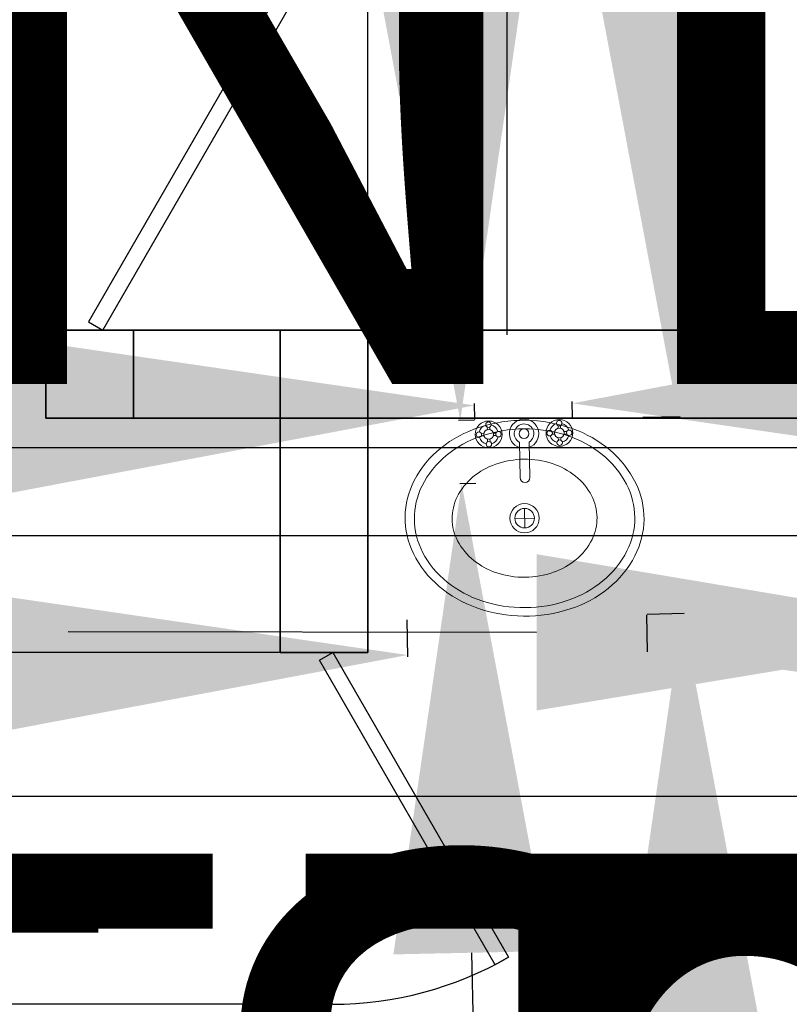
# Model space of a CAD drawing. Units: inches. Extents: x -307 to 2141, y -58 to 895.
# Tile 21 of 28: x 776 to 855, y 481 to 582. Entities that reach past the tile are written whole.
import ezdxf

# ---------------------------------------------------------------- set-up
doc = ezdxf.new("R2010")
doc.units = ezdxf.units.IN
doc.header["$MEASUREMENT"] = 0
for name, color, linetype, lineweight in [('A-ANNO-DIMS', 2, 'Continuous', 18), ('A-DOOR', 3, 'Continuous', 25), ('A-FLOR-FIXT', 9, 'Continuous', 18), ('A-WALL', 7, 'Continuous', 35)]:
    doc.layers.add(name, color=color, linetype=linetype, lineweight=lineweight)
doc.styles.get("Standard").update_dxf_attribs({"font": 'arial.ttf'})
doc.dimstyles.get("Standard").update_dxf_attribs({"dimtxt": 72, "dimasz": 48, "dimexe": 0.18, "dimexo": 0.0625, "dimgap": 0.09, "dimtad": 0, "dimtih": 1, "dimtoh": 1, "dimdec": 0, "dimrnd": 48, "dimzin": 0, "dimdsep": 46, "dimlunit": 3, "dimtxsty": 'Standard', "dimcen": 0.09, "dimadec": 0, "dimazin": 0, "dimtfac": 1, "dimtdec": 0, "dimtofl": 0, "dimtmove": 0, "dimatfit": 3, "dimfxl": 1, "dimtolj": 1, "dimtzin": 0, "dimarcsym": 0})

# ---------------------------------------------------------------- blocks, each defined once
blk = doc.blocks.new('*U2')
for p, q in [((0, 0), (0, -6)), ((-40, 0), (-40, -6))]:
    blk.add_line(p, q)
blk.add_lwpolyline([(0, 0), (-34.64, 20), (-35.52, 18.48), (-0.87, -1.52)], close=True)
blk.add_arc((0, 0), 40, 150, 180)
blk = doc.blocks.new('*U4')
for p, q in [((-40, 0), (-40, 6)), ((0, 0), (0, 6))]:
    blk.add_line(p, q)
blk.add_lwpolyline([(0, 0), (-34.64, -20), (-35.52, -18.48), (-0.88, 1.52)], close=True)
blk.add_arc((0, 0), 40, 180, 210)
blk = doc.blocks.new('Faucet - Bathroom top')
for p, q in [((-4.107, 0.125), (-4.375, 0.125)), ((-3.75, 0.4788), (-3.75, 0.75)), ((-3.5, 0.482), (-3.5, 0.75)), ((-3.1461, 0.125), (-2.875, 0.125)), ((3.143, 0.125), (2.875, 0.125)), ((3.5, 0.4788), (3.5, 0.75)), ((3.75, 0.482), (3.75, 0.75)), ((4.1039, 0.125), (4.375, 0.125)), ((-4.1039, -0.125), (-4.375, -0.125)), ((-3.75, -0.4821), (-3.75, -0.75)), ((-3.5, -0.4789), (-3.5, -0.75)), ((-3.143, -0.125), (-2.875, -0.125)), ((-0.5, -0.8639), (-0.5, -4.5)), ((0.5, -4.5), (0.5, -0.8631)), ((3.1461, -0.125), (2.875, -0.125)), ((3.5, -0.4821), (3.5, -0.75)), ((3.75, -0.4789), (3.75, -0.75)), ((4.107, -0.125), (4.375, -0.125))]:
    blk.add_line(p, q)
for centre, radius in [((-3.625, 0), 1.375), ((-3.625, 1), 0.2795), ((3.625, 0), 1.375), ((3.625, 1), 0.2795), ((-4.625, 0), 0.2795), ((-3.625, 0), 0.5), ((-2.625, 0), 0.2795), ((0, 0), 0.5), ((2.625, 0), 0.2795), ((3.625, 0), 0.5), ((4.625, 0), 0.2795), ((-3.625, -1), 0.2795), ((3.625, -1), 0.2795)]:
    blk.add_circle(centre, radius)
for centre, radius, start, end in [((0, 0), 1.5, 289.6514, 250.3603), ((-3.625, 0), 1, 105.2407, 164.2093), ((-3.625, 0), 1, 16.44125, 74.07887), ((0, 0), 1, 300.3431, 239.7554), ((3.625, 0), 1, 106.12, 164.0884), ((3.625, 0), 1, 16.23422, 73.90469), ((-3.625, 0), 1, 196.2342, 253.9047), ((-3.625, 0), 1, 286.12, 344.0884), ((3.625, 0), 1, 196.4413, 254.0789), ((3.625, 0), 1, 285.2407, 344.2093), ((0, -4.5), 0.5, 180, 0)]:
    blk.add_arc(centre, radius, start, end)
blk = doc.blocks.new('Sink - Oval top')
for p, q in [((-1, 0), (1, 0)), ((0, 1), (0, -1))]:
    blk.add_line(p, q)
for points in [[(-12.23, 0.39, 0.117634), (-11.46, -3.36, 0.104469), (-8.88, -6.8, 0.090016), (-5.08, -9.07, 0.08192), (-0.32, -10.02, 0.08192), (4.49, -9.38, 0.090016), (8.42, -7.36, 0.104469), (11.22, -4.09, 0.117634), (12.23, -0.39, 0.117634), (11.46, 3.36, 0.104469), (8.88, 6.8, 0.090016), (5.08, 9.07, 0.08192), (0.32, 10.02, 0.08192), (-4.49, 9.38, 0.090016), (-8.42, 7.36, 0.104469), (-11.22, 4.09, 0.117634)], [(-11.29, 0.16, 0.118622), (-10.52, -3.25, 0.104678), (-8.07, -6.36, 0.089562), (-4.54, -8.37, 0.081185), (-0.13, -9.15, 0.081185), (4.3, -8.49, 0.089562), (7.89, -6.58, 0.104678), (10.42, -3.55, 0.118622), (11.29, -0.16, 0.118622), (10.52, 3.25, 0.104678), (8.07, 6.36, 0.089562), (4.54, 8.37, 0.081185), (0.13, 9.15, 0.081185), (-4.3, 8.49, 0.089562), (-7.89, 6.58, 0.104678), (-10.42, 3.55, 0.118622)], [(-7.42, 0.08, 0.118283), (-6.91, -2.17, 0.104607), (-5.29, -4.21, 0.089718), (-2.97, -5.53, 0.081436), (-0.07, -6.04, 0.081436), (2.84, -5.59, 0.089718), (5.2, -4.33, 0.104607), (6.86, -2.32, 0.118283), (7.42, -0.08, 0.118283), (6.91, 2.17, 0.104607), (5.29, 4.21, 0.089718), (2.97, 5.53, 0.081436), (0.07, 6.04, 0.081436), (-2.84, 5.59, 0.089718), (-5.2, 4.33, 0.104607), (-6.86, 2.32, 0.118283)]]:
    blk.add_lwpolyline(points, format="xyb", close=True)
for radius in [1.5, 1]:
    blk.add_circle((0, 0), radius)
blk = doc.blocks.new('*D29')
at = {"layer": 'A-ANNO-DIMS', "color": 0, "lineweight": -2, "transparency": 16777216}
for p, q in [((747.42, 450.87), (699.42, 450.87)), ((795.42, 433.61), (795.42, 451.05)), ((882.03, 433.61), (882.03, 451.05)), ((930.03, 450.87), (978.03, 450.87))]:
    blk.add_line(p, q, dxfattribs=at)
at = {"layer": 'A-ANNO-DIMS', "color": 0, "transparency": 16777216}
for points in [[(747.42, 458.87), (747.42, 442.87), (795.42, 450.87)], [(930.03, 458.87), (930.03, 442.87), (882.03, 450.87)]]:
    blk.add_solid(points, dxfattribs=at)
at = {"layer": 'Defpoints', "color": 0, "transparency": 16777216}
for p in [(795.42, 450.87), (795.42, 433.55), (882.03, 433.55)]:
    blk.add_point(p, dxfattribs=at)
at = {"layer": 'A-ANNO-DIMS', "color": 0, "transparency": 16777216, "insert": (647.71, 450.87), "char_height": 72, "attachment_point": 5}
blk.add_mtext('\\A1;87', dxfattribs=at)
blk = doc.blocks.new('*D30')
at = {"layer": 'A-ANNO-DIMS', "color": 0, "lineweight": -2, "transparency": 16777216}
for p, q in [((570.74, 532.83), (570.74, 580.83)), ((570.74, 580.83), (618.74, 580.83)), ((565.4, 484.83), (570.92, 484.83)), ((565.4, 448.83), (570.92, 448.83)), ((570.74, 400.83), (570.74, 352.83))]:
    blk.add_line(p, q, dxfattribs=at)
at = {"layer": 'A-ANNO-DIMS', "color": 0, "transparency": 16777216}
for points in [[(562.74, 532.83), (578.74, 532.83), (570.74, 484.83)], [(562.74, 400.83), (578.74, 400.83), (570.74, 448.83)]]:
    blk.add_solid(points, dxfattribs=at)
at = {"layer": 'Defpoints', "color": 0, "transparency": 16777216}
for p in [(565.34, 484.83), (570.74, 484.83), (565.34, 448.83)]:
    blk.add_point(p, dxfattribs=at)
at = {"layer": 'A-ANNO-DIMS', "color": 0, "transparency": 16777216, "insert": (1030.17, 580.83), "char_height": 72, "attachment_point": 5}
blk.add_mtext('\\A1;WINDOW 36 TYP.', dxfattribs=at)
blk = doc.blocks.new('*D31')
at = {"layer": 'A-ANNO-DIMS', "color": 0, "lineweight": -2, "transparency": 16777216}
for p, q in [((556.34, 448.77), (556.34, 443.25)), ((565.34, 448.77), (565.34, 443.25)), ((508.34, 443.43), (460.34, 443.43)), ((613.34, 443.43), (661.34, 443.43))]:
    blk.add_line(p, q, dxfattribs=at)
at = {"layer": 'A-ANNO-DIMS', "color": 0, "transparency": 16777216}
for points in [[(508.34, 451.43), (508.34, 435.43), (556.34, 443.43)], [(613.34, 451.43), (613.34, 435.43), (565.34, 443.43)]]:
    blk.add_solid(points, dxfattribs=at)
at = {"layer": 'Defpoints', "color": 0, "transparency": 16777216}
for p in [(556.34, 448.83), (565.34, 448.83), (565.34, 443.43)]:
    blk.add_point(p, dxfattribs=at)
at = {"layer": 'A-ANNO-DIMS', "color": 0, "transparency": 16777216, "insert": (808.69, 443.43), "char_height": 72, "attachment_point": 5}
blk.add_mtext('\\A1;9 TYP.', dxfattribs=at)
blk = doc.blocks.new('*D32')
at = {"layer": 'A-ANNO-DIMS', "color": 0, "lineweight": -2, "transparency": 16777216}
for p, q in [((813.29, 682.28), (813.29, 671.36)), ((885.29, 682.28), (885.29, 671.36)), ((765.29, 671.54), (717.29, 671.54)), ((933.29, 671.54), (981.29, 671.54))]:
    blk.add_line(p, q, dxfattribs=at)
at = {"layer": 'A-ANNO-DIMS', "color": 0, "transparency": 16777216}
for points in [[(765.29, 679.54), (765.29, 663.54), (813.29, 671.54)], [(933.29, 679.54), (933.29, 663.54), (885.29, 671.54)]]:
    blk.add_solid(points, dxfattribs=at)
at = {"layer": 'Defpoints', "color": 0, "transparency": 16777216}
for p in [(813.29, 682.34), (885.29, 682.34), (885.29, 671.54)]:
    blk.add_point(p, dxfattribs=at)
at = {"layer": 'A-ANNO-DIMS', "color": 0, "transparency": 16777216, "insert": (1392.73, 671.54), "char_height": 72, "attachment_point": 5}
blk.add_mtext('\\A1;WINDOW 72 TYP.', dxfattribs=at)
blk = doc.blocks.new('*D35')
at = {"layer": 'A-ANNO-DIMS', "color": 0, "lineweight": -2, "transparency": 16777216}
for p, q in [((859.34, 453.77), (811.34, 453.77)), ((907.34, 443.03), (907.34, 453.95)), ((916.34, 443.03), (916.34, 453.95)), ((964.34, 453.77), (1012.34, 453.77))]:
    blk.add_line(p, q, dxfattribs=at)
at = {"layer": 'A-ANNO-DIMS', "color": 0, "transparency": 16777216}
for points in [[(859.34, 461.77), (859.34, 445.77), (907.34, 453.77)], [(964.34, 461.77), (964.34, 445.77), (916.34, 453.77)]]:
    blk.add_solid(points, dxfattribs=at)
at = {"layer": 'Defpoints', "color": 0, "transparency": 16777216}
for p in [(907.34, 453.77), (907.34, 442.97), (916.34, 442.97)]:
    blk.add_point(p, dxfattribs=at)
at = {"layer": 'A-ANNO-DIMS', "color": 0, "transparency": 16777216, "insert": (663.98, 453.77), "char_height": 72, "attachment_point": 5}
blk.add_mtext('\\A1;9 TYP.', dxfattribs=at)
blk = doc.blocks.new('*D36')
at = {"layer": 'A-ANNO-DIMS', "color": 0, "lineweight": -2, "transparency": 16777216}
for p, q in [((871.71, 562.4), (871.76, 610.4)), ((876.55, 514.4), (871.47, 514.4)), ((876.51, 481.35), (871.44, 481.36)), ((871.56, 433.36), (871.51, 385.36)), ((871.51, 385.36), (823.51, 385.36))]:
    blk.add_line(p, q, dxfattribs=at)
at = {"layer": 'A-ANNO-DIMS', "color": 0, "transparency": 16777216}
for points in [[(863.71, 562.41), (879.71, 562.4), (871.65, 514.4)], [(863.56, 433.37), (879.56, 433.35), (871.62, 481.36)]]:
    blk.add_solid(points, dxfattribs=at)
at = {"layer": 'Defpoints', "color": 0, "transparency": 16777216}
for p in [(876.61, 514.4), (871.62, 481.36), (876.57, 481.35)]:
    blk.add_point(p, dxfattribs=at)
at = {"layer": 'A-ANNO-DIMS', "color": 0, "transparency": 16777216, "insert": (548.95, 385.36), "char_height": 72, "attachment_point": 5}
blk.add_mtext('\\A1;WC 33 TYP.', dxfattribs=at)
blk = doc.blocks.new('*D37')
at = {"layer": 'A-ANNO-DIMS', "color": 0, "lineweight": -2, "transparency": 16777216}
for p, q in [((828.62, 519.41), (780.62, 519.46)), ((876.61, 514.46), (876.62, 519.54)), ((897.61, 514.44), (897.62, 519.51)), ((945.62, 519.28), (993.62, 519.22))]:
    blk.add_line(p, q, dxfattribs=at)
at = {"layer": 'A-ANNO-DIMS', "color": 0, "transparency": 16777216}
for points in [[(828.63, 527.41), (828.61, 511.41), (876.62, 519.36)], [(945.63, 527.28), (945.61, 511.28), (897.62, 519.33)]]:
    blk.add_solid(points, dxfattribs=at)
at = {"layer": 'Defpoints', "color": 0, "transparency": 16777216}
for p in [(876.62, 519.36), (876.61, 514.4), (897.61, 514.38)]:
    blk.add_point(p, dxfattribs=at)
at = {"layer": 'A-ANNO-DIMS', "color": 0, "transparency": 16777216, "insert": (604.68, 519.46), "char_height": 72, "attachment_point": 5}
blk.add_mtext('\\A1;21 TYP.', dxfattribs=at)
blk = doc.blocks.new('*D42')
at = {"layer": 'A-ANNO-DIMS', "color": 0, "lineweight": -2, "transparency": 16777216}
for p, q in [((880.26, 543.86), (928.25, 544.87)), ((822.3, 541.2), (822.27, 542.82)), ((832.3, 541.41), (832.27, 543.03)), ((774.28, 541.63), (726.29, 540.62))]:
    blk.add_line(p, q, dxfattribs=at)
at = {"layer": 'A-ANNO-DIMS', "color": 0, "transparency": 16777216}
for points in [[(880.09, 551.86), (880.43, 535.86), (832.27, 542.85)], [(774.11, 549.63), (774.45, 533.63), (822.27, 542.64)]]:
    blk.add_solid(points, dxfattribs=at)
at = {"layer": 'Defpoints', "color": 0, "transparency": 16777216}
for p in [(832.27, 542.85), (832.3, 541.35), (822.3, 541.14)]:
    blk.add_point(p, dxfattribs=at)
at = {"layer": 'A-ANNO-DIMS', "color": 0, "transparency": 16777216, "insert": (1192.89, 544.87), "char_height": 72, "attachment_point": 5}
blk.add_mtext('\\A1;FAUCET 10', dxfattribs=at)
blk = doc.blocks.new('*D43')
at = {"layer": 'A-ANNO-DIMS', "color": 0, "lineweight": -2, "transparency": 16777216}
for p, q in [((818.79, 637.09), (770.79, 637.09)), ((819.79, 589.1), (818.79, 637.09)), ((822.24, 541.14), (820.62, 541.1)), ((822.38, 534.64), (820.76, 534.61)), ((821.95, 486.62), (822.96, 438.63))]:
    blk.add_line(p, q, dxfattribs=at)
at = {"layer": 'A-ANNO-DIMS', "color": 0, "transparency": 16777216}
for points in [[(827.79, 589.27), (811.8, 588.93), (820.8, 541.11)], [(829.95, 486.79), (813.95, 486.45), (820.94, 534.61)]]:
    blk.add_solid(points, dxfattribs=at)
at = {"layer": 'Defpoints', "color": 0, "transparency": 16777216}
for p in [(820.8, 541.11), (822.3, 541.14), (822.44, 534.64)]:
    blk.add_point(p, dxfattribs=at)
at = {"layer": 'A-ANNO-DIMS', "color": 0, "transparency": 16777216, "insert": (747.39, 637.09), "char_height": 72, "attachment_point": 5}
blk.add_mtext('\\A1;7', dxfattribs=at)
blk = doc.blocks.new('*D44')
at = {"layer": 'A-ANNO-DIMS', "color": 0, "lineweight": -2, "transparency": 16777216}
for p, q in [((839.87, 521.22), (839.95, 517.42)), ((815.33, 520.71), (815.41, 516.91)), ((887.94, 518.61), (935.93, 519.62)), ((767.41, 516.08), (719.42, 515.07))]:
    blk.add_line(p, q, dxfattribs=at)
at = {"layer": 'A-ANNO-DIMS', "color": 0, "transparency": 16777216}
for points in [[(887.77, 526.61), (888.11, 510.61), (839.95, 517.6)], [(767.25, 524.08), (767.58, 508.08), (815.4, 517.09)]]:
    blk.add_solid(points, dxfattribs=at)
at = {"layer": 'Defpoints', "color": 0, "transparency": 16777216}
for p in [(839.87, 521.29), (815.33, 520.77), (839.95, 517.6)]:
    blk.add_point(p, dxfattribs=at)
at = {"layer": 'A-ANNO-DIMS', "color": 0, "transparency": 16777216, "insert": (1151.16, 519.62), "char_height": 72, "attachment_point": 5}
blk.add_mtext('\\A1;BASIN 25', dxfattribs=at)
blk = doc.blocks.new('*D45')
at = {"layer": 'A-ANNO-DIMS', "color": 0, "lineweight": -2, "transparency": 16777216}
for p, q in [((841.11, 637.47), (793.11, 637.47)), ((842.12, 589.48), (841.11, 637.47)), ((839.51, 541.42), (843.31, 541.5)), ((839.93, 521.29), (843.73, 521.37)), ((844.56, 473.37), (845.57, 425.38))]:
    blk.add_line(p, q, dxfattribs=at)
at = {"layer": 'A-ANNO-DIMS', "color": 0, "transparency": 16777216}
for points in [[(850.12, 589.65), (834.12, 589.32), (843.13, 541.49)], [(852.56, 473.54), (836.56, 473.21), (843.55, 521.36)]]:
    blk.add_solid(points, dxfattribs=at)
at = {"layer": 'Defpoints', "color": 0, "transparency": 16777216}
for p in [(839.45, 541.42), (843.13, 541.49), (839.87, 521.29)]:
    blk.add_point(p, dxfattribs=at)
at = {"layer": 'A-ANNO-DIMS', "color": 0, "transparency": 16777216, "insert": (740.96, 637.47), "char_height": 72, "attachment_point": 5}
blk.add_mtext('\\A1;20', dxfattribs=at)
blk = doc.blocks.new('*D46')
at = {"layer": 'A-ANNO-DIMS', "color": 0, "lineweight": -2, "transparency": 16777216}
for p, q in [((801.41, 645.78), (801.41, 642.52)), ((822.41, 645.78), (822.41, 642.52)), ((753.41, 642.7), (705.41, 642.7)), ((870.41, 642.7), (918.41, 642.7))]:
    blk.add_line(p, q, dxfattribs=at)
at = {"layer": 'A-ANNO-DIMS', "color": 0, "transparency": 16777216}
for points in [[(753.41, 650.7), (753.41, 634.7), (801.41, 642.7)], [(870.41, 650.7), (870.41, 634.7), (822.41, 642.7)]]:
    blk.add_solid(points, dxfattribs=at)
at = {"layer": 'Defpoints', "color": 0, "transparency": 16777216}
for p in [(801.41, 645.85), (822.41, 645.85), (822.41, 642.7)]:
    blk.add_point(p, dxfattribs=at)
at = {"layer": 'A-ANNO-DIMS', "color": 0, "transparency": 16777216, "insert": (1282.7, 642.7), "char_height": 72, "attachment_point": 5}
blk.add_mtext('\\A1;DESK CHAIR 21', dxfattribs=at)
blk = doc.blocks.new('*D47')
at = {"layer": 'A-ANNO-DIMS', "color": 0, "lineweight": -2, "transparency": 16777216}
for p, q in [((825.56, 711.18), (825.56, 759.18)), ((825.56, 759.18), (873.56, 759.18)), ((822.48, 663.18), (825.74, 663.18)), ((822.48, 645.85), (825.74, 645.85)), ((825.56, 597.85), (825.56, 549.85))]:
    blk.add_line(p, q, dxfattribs=at)
at = {"layer": 'A-ANNO-DIMS', "color": 0, "transparency": 16777216}
for points in [[(817.56, 711.18), (833.56, 711.18), (825.56, 663.18)], [(817.56, 597.85), (833.56, 597.85), (825.56, 645.85)]]:
    blk.add_solid(points, dxfattribs=at)
at = {"layer": 'Defpoints', "color": 0, "transparency": 16777216}
for p in [(822.41, 663.18), (825.56, 663.18), (822.41, 645.85)]:
    blk.add_point(p, dxfattribs=at)
at = {"layer": 'A-ANNO-DIMS', "color": 0, "transparency": 16777216, "insert": (921.83, 759.18), "char_height": 72, "attachment_point": 5}
blk.add_mtext('\\A1;17', dxfattribs=at)
blk = doc.blocks.new('*D52')
at = {"layer": 'A-ANNO-DIMS', "color": 0, "lineweight": -2, "transparency": 16777216}
for p, q in [((660.21, 554.25), (660.21, 602.25)), ((673.8, 506.25), (660.03, 506.25)), ((673.8, 415.25), (660.03, 415.25)), ((660.21, 367.25), (660.21, 319.25))]:
    blk.add_line(p, q, dxfattribs=at)
at = {"layer": 'A-ANNO-DIMS', "color": 0, "transparency": 16777216}
for points in [[(652.21, 554.25), (668.21, 554.25), (660.21, 506.25)], [(652.21, 367.25), (668.21, 367.25), (660.21, 415.25)]]:
    blk.add_solid(points, dxfattribs=at)
at = {"layer": 'Defpoints', "color": 0, "transparency": 16777216}
for p in [(673.86, 506.25), (660.21, 415.25), (673.86, 415.25)]:
    blk.add_point(p, dxfattribs=at)
at = {"layer": 'A-ANNO-DIMS', "color": 0, "transparency": 16777216, "insert": (660.21, 460.75), "char_height": 72, "attachment_point": 5}
blk.add_mtext('\\A1;DINING SET 91', dxfattribs=at)
blk = doc.blocks.new('*D54')
at = {"layer": 'A-ANNO-DIMS', "color": 0, "lineweight": -2, "transparency": 16777216}
for p, q in [((605.34, 412.35), (605.34, 460.35)), ((605.34, 460.35), (653.34, 460.35)), ((596.4, 364.35), (605.52, 364.35)), ((596.4, 304.35), (605.52, 304.35)), ((605.34, 256.35), (605.34, 208.35))]:
    blk.add_line(p, q, dxfattribs=at)
at = {"layer": 'A-ANNO-DIMS', "color": 0, "transparency": 16777216}
for points in [[(597.34, 412.35), (613.34, 412.35), (605.34, 364.35)], [(597.34, 256.35), (613.34, 256.35), (605.34, 304.35)]]:
    blk.add_solid(points, dxfattribs=at)
at = {"layer": 'Defpoints', "color": 0, "transparency": 16777216}
for p in [(596.34, 364.35), (605.34, 364.35), (596.34, 304.35)]:
    blk.add_point(p, dxfattribs=at)
at = {"layer": 'A-ANNO-DIMS', "color": 0, "transparency": 16777216, "insert": (854, 460.35), "char_height": 72, "attachment_point": 5}
blk.add_mtext('\\A1;DESK 60', dxfattribs=at)
blk = doc.blocks.new('*D56')
at = {"layer": 'A-ANNO-DIMS', "color": 0, "lineweight": -2, "transparency": 16777216}
for p, q in [((679.73, 723.21), (679.73, 771.21)), ((679.73, 771.21), (727.73, 771.21)), ((675.74, 675.21), (679.91, 675.21)), ((675.74, 648.21), (679.91, 648.21)), ((679.73, 600.21), (679.73, 552.21))]:
    blk.add_line(p, q, dxfattribs=at)
at = {"layer": 'A-ANNO-DIMS', "color": 0, "transparency": 16777216}
for points in [[(671.73, 723.21), (687.73, 723.21), (679.73, 675.21)], [(671.73, 600.21), (687.73, 600.21), (679.73, 648.21)]]:
    blk.add_solid(points, dxfattribs=at)
at = {"layer": 'Defpoints', "color": 0, "transparency": 16777216}
for p in [(675.68, 675.21), (679.73, 675.21), (675.68, 648.21)]:
    blk.add_point(p, dxfattribs=at)
at = {"layer": 'A-ANNO-DIMS', "color": 0, "transparency": 16777216, "insert": (1006.66, 771.21), "char_height": 72, "attachment_point": 5}
blk.add_mtext('\\A1;ROCKER 27', dxfattribs=at)
blk = doc.blocks.new('*D62')
at = {"layer": 'A-ANNO-DIMS', "color": 0, "lineweight": -2, "transparency": 16777216}
for p, q in [((556.34, 691.4), (556.34, 722.72)), ((916.34, 490.97), (916.34, 722.72)), ((604.34, 722.54), (656.85, 722.54)), ((868.34, 722.54), (815.82, 722.54))]:
    blk.add_line(p, q, dxfattribs=at)
at = {"layer": 'A-ANNO-DIMS', "color": 0, "transparency": 16777216}
for points in [[(604.34, 730.54), (604.34, 714.54), (556.34, 722.54)], [(868.34, 730.54), (868.34, 714.54), (916.34, 722.54)]]:
    blk.add_solid(points, dxfattribs=at)
at = {"layer": 'Defpoints', "color": 0, "transparency": 16777216}
for p in [(916.34, 722.54), (556.34, 691.34), (916.34, 490.9)]:
    blk.add_point(p, dxfattribs=at)
at = {"layer": 'A-ANNO-DIMS', "color": 0, "transparency": 16777216, "insert": (736.34, 722.54), "char_height": 72, "attachment_point": 5}
blk.add_mtext('\\A1;360', dxfattribs=at)
blk = doc.blocks.new('*D63')
at = {"layer": 'A-ANNO-DIMS', "color": 0, "lineweight": -2, "transparency": 16777216}
for p, q in [((916.4, 691.34), (947.72, 691.34)), ((947.54, 643.34), (947.54, 416.19)), ((947.54, 115.34), (947.54, 342.49)), ((704.68, 67.34), (947.72, 67.34))]:
    blk.add_line(p, q, dxfattribs=at)
at = {"layer": 'A-ANNO-DIMS', "color": 0, "transparency": 16777216}
for points in [[(939.54, 643.34), (955.54, 643.34), (947.54, 691.34)], [(939.54, 115.34), (955.54, 115.34), (947.54, 67.34)]]:
    blk.add_solid(points, dxfattribs=at)
at = {"layer": 'Defpoints', "color": 0, "transparency": 16777216}
for p in [(916.34, 691.34), (704.62, 67.34), (947.54, 67.34)]:
    blk.add_point(p, dxfattribs=at)
at = {"layer": 'A-ANNO-DIMS', "color": 0, "transparency": 16777216, "insert": (947.54, 379.34), "char_height": 72, "attachment_point": 5}
blk.add_mtext('\\A1;624', dxfattribs=at)
blk = doc.blocks.new('*D68')
at = {"layer": 'A-ANNO-DIMS', "color": 0, "lineweight": -2, "transparency": 16777216}
for p, q in [((525.13, 586.34), (525.13, 634.34)), ((525.13, 634.34), (573.13, 634.34)), ((565.27, 538.34), (524.95, 538.34)), ((556.27, 484.83), (524.95, 484.83)), ((525.13, 436.83), (525.13, 388.83))]:
    blk.add_line(p, q, dxfattribs=at)
at = {"layer": 'A-ANNO-DIMS', "color": 0, "transparency": 16777216}
for points in [[(517.13, 586.34), (533.13, 586.34), (525.13, 538.34)], [(517.13, 436.83), (533.13, 436.83), (525.13, 484.83)]]:
    blk.add_solid(points, dxfattribs=at)
at = {"layer": 'Defpoints', "color": 0, "transparency": 16777216}
for p in [(525.13, 538.34), (565.34, 538.34), (556.34, 484.83)]:
    blk.add_point(p, dxfattribs=at)
at = {"layer": 'A-ANNO-DIMS', "color": 0, "transparency": 16777216, "insert": (687.75, 634.34), "char_height": 72, "attachment_point": 5}
blk.add_mtext('\\A1;53.51', dxfattribs=at)
blk = doc.blocks.new('*D78')
at = {"layer": 'A-ANNO-DIMS', "color": 0, "lineweight": -2, "transparency": 16777216}
for p, q in [((947.53984, 730.340828), (947.53984, 778.340828)), ((778.39834, 682.340828), (947.71984, 682.340828)), ((730.39834, 598.340828), (947.71984, 598.340828)), ((947.53984, 550.340828), (947.53984, 502.340828))]:
    blk.add_line(p, q, dxfattribs=at)
at = {"layer": 'A-ANNO-DIMS', "color": 0, "transparency": 16777216}
for points in [[(939.53984, 730.340828), (955.53984, 730.340828), (947.53984, 682.340828)], [(939.53984, 550.340828), (955.53984, 550.340828), (947.53984, 598.340828)]]:
    blk.add_solid(points, dxfattribs=at)
at = {"layer": 'Defpoints', "color": 0, "transparency": 16777216}
for p in [(778.33584, 682.340828), (947.53984, 682.340828), (730.33584, 598.340828)]:
    blk.add_point(p, dxfattribs=at)
at = {"layer": 'A-ANNO-DIMS', "color": 0, "transparency": 16777216, "insert": (947.53984, 640.340828), "char_height": 72, "attachment_point": 5}
blk.add_mtext('\\A1;84', dxfattribs=at)
blk = doc.blocks.new('*D80')
at = {"layer": 'A-ANNO-DIMS', "color": 0, "lineweight": -2, "transparency": 16777216}
for p, q in [((811.34, 517.4), (811.34, 722.72)), ((907.34, 541.4), (907.34, 722.72)), ((763.34, 722.54), (715.34, 722.54)), ((955.34, 722.54), (1003.34, 722.54))]:
    blk.add_line(p, q, dxfattribs=at)
at = {"layer": 'A-ANNO-DIMS', "color": 0, "transparency": 16777216}
for points in [[(763.34, 730.54), (763.34, 714.54), (811.34, 722.54)], [(955.34, 730.54), (955.34, 714.54), (907.34, 722.54)]]:
    blk.add_solid(points, dxfattribs=at)
at = {"layer": 'Defpoints', "color": 0, "transparency": 16777216}
for p in [(907.34, 722.54), (907.34, 541.34), (811.34, 517.34)]:
    blk.add_point(p, dxfattribs=at)
at = {"layer": 'A-ANNO-DIMS', "color": 0, "transparency": 16777216, "insert": (1054.97, 722.54), "char_height": 72, "attachment_point": 5}
blk.add_mtext('\\A1;96', dxfattribs=at)
blk = doc.blocks.new('*D82')
at = {"layer": 'A-ANNO-DIMS', "color": 0, "lineweight": -2, "transparency": 16777216}
for p, q in [((525.13, 565.34), (525.13, 613.34)), ((525.13, 613.34), (573.13, 613.34)), ((802.27, 517.34), (524.95, 517.34)), ((802.27, 481.34), (524.95, 481.34)), ((525.13, 433.34), (525.13, 385.34))]:
    blk.add_line(p, q, dxfattribs=at)
at = {"layer": 'A-ANNO-DIMS', "color": 0, "transparency": 16777216}
for points in [[(517.13, 565.34), (533.13, 565.34), (525.13, 517.34)], [(517.13, 433.34), (533.13, 433.34), (525.13, 481.34)]]:
    blk.add_solid(points, dxfattribs=at)
at = {"layer": 'Defpoints', "color": 0, "transparency": 16777216}
for p in [(525.13, 517.34), (802.34, 517.34), (802.34, 481.34)]:
    blk.add_point(p, dxfattribs=at)
at = {"layer": 'A-ANNO-DIMS', "color": 0, "transparency": 16777216, "insert": (624.74, 613.34), "char_height": 72, "attachment_point": 5}
blk.add_mtext('\\A1;36', dxfattribs=at)
blk = doc.blocks.new('*D83')
at = {"layer": 'A-ANNO-DIMS', "color": 0, "lineweight": -2, "transparency": 16777216}
for p, q in [((947.54, 538.9), (947.54, 586.9)), ((916.4, 490.9), (947.72, 490.9)), ((907.4, 481.34), (947.72, 481.34)), ((947.54, 433.34), (947.54, 385.34)), ((947.54, 385.34), (899.54, 385.34))]:
    blk.add_line(p, q, dxfattribs=at)
at = {"layer": 'A-ANNO-DIMS', "color": 0, "transparency": 16777216}
for points in [[(939.54, 538.9), (955.54, 538.9), (947.54, 490.9)], [(939.54, 433.34), (955.54, 433.34), (947.54, 481.34)]]:
    blk.add_solid(points, dxfattribs=at)
at = {"layer": 'Defpoints', "color": 0, "transparency": 16777216}
for p in [(916.34, 490.9), (907.34, 481.34), (947.54, 481.34)]:
    blk.add_point(p, dxfattribs=at)
at = {"layer": 'A-ANNO-DIMS', "color": 0, "transparency": 16777216, "insert": (777.97, 385.34), "char_height": 72, "attachment_point": 5}
blk.add_mtext('\\A1;9.563', dxfattribs=at)
blk = doc.blocks.new('*D88')
at = {"layer": 'A-ANNO-DIMS', "color": 0, "lineweight": -2, "transparency": 16777216}
for p, q in [((565.33584, 295.403328), (565.33584, 722.724828)), ((754.33584, 271.403328), (754.33584, 722.724828)), ((517.33584, 722.544828), (469.33584, 722.544828)), ((802.33584, 722.544828), (850.33584, 722.544828))]:
    blk.add_line(p, q, dxfattribs=at)
at = {"layer": 'A-ANNO-DIMS', "color": 0, "transparency": 16777216}
for points in [[(517.33584, 730.544828), (517.33584, 714.544828), (565.33584, 722.544828)], [(802.33584, 730.544828), (802.33584, 714.544828), (754.33584, 722.544828)]]:
    blk.add_solid(points, dxfattribs=at)
at = {"layer": 'Defpoints', "color": 0, "transparency": 16777216}
for p in [(754.33584, 722.544828), (565.33584, 295.340828), (754.33584, 271.340828)]:
    blk.add_point(p, dxfattribs=at)
at = {"layer": 'A-ANNO-DIMS', "color": 0, "transparency": 16777216, "insert": (659.83584, 722.544828), "char_height": 72, "attachment_point": 5}
blk.add_mtext('\\A1;189', dxfattribs=at)
blk = doc.blocks.new('*D94')
at = {"layer": 'A-ANNO-DIMS', "color": 0, "lineweight": -2, "transparency": 16777216}
for p, q in [((565.34, 529.4), (565.34, 722.72)), ((629.84, 529.4), (629.84, 722.72)), ((517.34, 722.54), (469.34, 722.54)), ((677.84, 722.54), (725.84, 722.54))]:
    blk.add_line(p, q, dxfattribs=at)
at = {"layer": 'A-ANNO-DIMS', "color": 0, "transparency": 16777216}
for points in [[(517.34, 730.54), (517.34, 714.54), (565.34, 722.54)], [(677.84, 730.54), (677.84, 714.54), (629.84, 722.54)]]:
    blk.add_solid(points, dxfattribs=at)
at = {"layer": 'Defpoints', "color": 0, "transparency": 16777216}
for p in [(629.84, 722.54), (565.34, 529.34), (629.84, 529.34)]:
    blk.add_point(p, dxfattribs=at)
at = {"layer": 'A-ANNO-DIMS', "color": 0, "transparency": 16777216, "insert": (819.9, 722.54), "char_height": 72, "attachment_point": 5}
blk.add_mtext('\\A1;64.5', dxfattribs=at)
blk = doc.blocks.new('*D95')
at = {"layer": 'A-ANNO-DIMS', "color": 0, "lineweight": -2, "transparency": 16777216}
for p, q in [((947.54, 577.34), (947.54, 625.34)), ((947.54, 625.34), (995.54, 625.34)), ((629.9, 529.34), (947.72, 529.34)), ((629.9, 502.66), (947.72, 502.66)), ((947.54, 454.66), (947.54, 406.66))]:
    blk.add_line(p, q, dxfattribs=at)
at = {"layer": 'A-ANNO-DIMS', "color": 0, "transparency": 16777216}
for points in [[(939.54, 577.34), (955.54, 577.34), (947.54, 529.34)], [(939.54, 454.66), (955.54, 454.66), (947.54, 502.66)]]:
    blk.add_solid(points, dxfattribs=at)
at = {"layer": 'Defpoints', "color": 0, "transparency": 16777216}
for p in [(629.84, 529.34), (947.54, 529.34), (629.84, 502.66)]:
    blk.add_point(p, dxfattribs=at)
at = {"layer": 'A-ANNO-DIMS', "color": 0, "transparency": 16777216, "insert": (1117.8, 625.34), "char_height": 72, "attachment_point": 5}
blk.add_mtext('\\A1;26.68', dxfattribs=at)
blk = doc.blocks.new('*D97')
at = {"layer": 'A-ANNO-DIMS', "color": 0, "lineweight": -2, "transparency": 16777216}
for p, q in [((947.54, 637.34), (947.54, 685.34)), ((947.54, 685.34), (995.54, 685.34)), ((685.4, 589.34), (947.72, 589.34)), ((685.4, 538.34), (947.72, 538.34)), ((947.54, 490.34), (947.54, 442.34))]:
    blk.add_line(p, q, dxfattribs=at)
at = {"layer": 'A-ANNO-DIMS', "color": 0, "transparency": 16777216}
for points in [[(939.54, 637.34), (955.54, 637.34), (947.54, 589.34)], [(939.54, 490.34), (955.54, 490.34), (947.54, 538.34)]]:
    blk.add_solid(points, dxfattribs=at)
at = {"layer": 'Defpoints', "color": 0, "transparency": 16777216}
for p in [(685.34, 589.34), (947.54, 589.34), (685.34, 538.34)]:
    blk.add_point(p, dxfattribs=at)
at = {"layer": 'A-ANNO-DIMS', "color": 0, "transparency": 16777216, "insert": (1040.25, 685.34), "char_height": 72, "attachment_point": 5}
blk.add_mtext('\\A1;51', dxfattribs=at)
blk = doc.blocks.new('*D98')
at = {"layer": 'A-ANNO-DIMS', "color": 0, "lineweight": -2, "transparency": 16777216}
for p, q in [((525.13, 637.34), (525.13, 685.34)), ((525.13, 685.34), (573.13, 685.34)), ((787.27, 589.34), (524.95, 589.34)), ((787.27, 550.34), (524.95, 550.34)), ((525.13, 502.34), (525.13, 454.34))]:
    blk.add_line(p, q, dxfattribs=at)
at = {"layer": 'A-ANNO-DIMS', "color": 0, "transparency": 16777216}
for points in [[(517.13, 637.34), (533.13, 637.34), (525.13, 589.34)], [(517.13, 502.34), (533.13, 502.34), (525.13, 550.34)]]:
    blk.add_solid(points, dxfattribs=at)
at = {"layer": 'Defpoints', "color": 0, "transparency": 16777216}
for p in [(525.13, 589.34), (787.34, 589.34), (787.34, 550.34)]:
    blk.add_point(p, dxfattribs=at)
at = {"layer": 'A-ANNO-DIMS', "color": 0, "transparency": 16777216, "insert": (624.84, 685.34), "char_height": 72, "attachment_point": 5}
blk.add_mtext('\\A1;39', dxfattribs=at)
blk = doc.blocks.new('*D107')
at = {"layer": 'A-ANNO-DIMS', "color": 0, "lineweight": -2, "transparency": 16777216}
for p, q in [((565.34, 409.4), (565.34, 722.72)), ((589.34, 409.4), (589.34, 722.72)), ((517.34, 722.54), (469.34, 722.54)), ((637.34, 722.54), (685.34, 722.54))]:
    blk.add_line(p, q, dxfattribs=at)
at = {"layer": 'A-ANNO-DIMS', "color": 0, "transparency": 16777216}
for points in [[(517.34, 730.54), (517.34, 714.54), (565.34, 722.54)], [(637.34, 730.54), (637.34, 714.54), (589.34, 722.54)]]:
    blk.add_solid(points, dxfattribs=at)
at = {"layer": 'Defpoints', "color": 0, "transparency": 16777216}
for p in [(589.34, 722.54), (565.34, 409.34), (589.34, 409.34)]:
    blk.add_point(p, dxfattribs=at)
at = {"layer": 'A-ANNO-DIMS', "color": 0, "transparency": 16777216, "insert": (835.49, 722.54), "char_height": 72, "attachment_point": 5}
blk.add_mtext('\\A1;24.003', dxfattribs=at)
blk = doc.blocks.new('*D108')
at = {"layer": 'A-ANNO-DIMS', "color": 0, "lineweight": -2, "transparency": 16777216}
for p, q in [((947.54, 550.66), (947.54, 598.66)), ((589.4, 502.66), (947.72, 502.66)), ((589.4, 409.34), (947.72, 409.34)), ((947.54, 361.34), (947.54, 313.34))]:
    blk.add_line(p, q, dxfattribs=at)
at = {"layer": 'A-ANNO-DIMS', "color": 0, "transparency": 16777216}
for points in [[(939.54, 550.66), (955.54, 550.66), (947.54, 502.66)], [(939.54, 361.34), (955.54, 361.34), (947.54, 409.34)]]:
    blk.add_solid(points, dxfattribs=at)
at = {"layer": 'Defpoints', "color": 0, "transparency": 16777216}
for p in [(589.34, 502.66), (947.54, 502.66), (589.34, 409.34)]:
    blk.add_point(p, dxfattribs=at)
at = {"layer": 'A-ANNO-DIMS', "color": 0, "transparency": 16777216, "insert": (947.54, 456), "char_height": 72, "attachment_point": 5}
blk.add_mtext('\\A1;93.32', dxfattribs=at)

msp = doc.modelspace()

# ---------------------------------------------------------------- linework, layer by layer
at = {"layer": 'A-WALL'}
for p, q in [((778.3358, 541.3408), (778.3358, 550.3408)), ((907.3358, 550.3408), (778.3358, 550.3408)), ((787.3358, 541.3408), (787.3358, 550.3408)), ((802.3358, 517.3408), (802.3358, 550.3408)), ((811.3358, 517.3408), (811.3358, 550.3408)), ((907.3358, 541.3408), (778.3358, 541.3408)), ((811.3358, 517.3408), (802.3358, 517.3408))]:
    msp.add_line(p, q, dxfattribs=at)

# ---------------------------------------------------------------- block references
at = {"layer": 'A-DOOR'}
for name, p, xscale, yscale, zscale, rotation in [('*U2', (784.1958, 550.3408), 0.9766664716736615, 0.9766664716736615, 0.9766664716736615, 270), ('*U4', (807.7357, 517.3408), 0.8999759086529358, 0.8999759086529358, 0.8999759086529358, 89.99999999999996)]:
    msp.add_blockref(name, p, dxfattribs=dict(at, xscale=xscale, yscale=yscale, zscale=zscale, rotation=rotation))
at = {"layer": 'A-FLOR-FIXT', "rotation": 1.204627671485523}
for name, p in [('Sink - Oval top', (827.3863, 531.0933)), ('Faucet - Bathroom top', (827.3334, 539.7456))]:
    msp.add_blockref(name, p, dxfattribs=at)

# ---------------------------------------------------------------- dimensions: what is measured, and where the dimension line sits
at = {"layer": 'A-ANNO-DIMS'}
for base, p1, p2, angle, text, picture, middle in [((679.7317, 675.211), (675.6817, 648.211), (675.6817, 675.211), 90, 'ROCKER <>', '*D56', (1006.6621, 771.211)), ((570.7358, 484.8333), (565.3358, 448.8333), (565.3358, 484.8333), 90, 'WINDOW <> TYP.', '*D30', (1030.1737, 580.8333)), ((832.2692, 542.8502), (822.3029, 541.1403), (832.3007, 541.3505), 1.204628, 'FAUCET <>', '*D42', (1192.8864, 544.8684)), ((660.2083, 415.2485), (673.8583, 506.2485), (673.8583, 415.2485), 270, 'DINING SET <>', '*D52', (660.2083, 460.7485)), ((839.9481, 517.6035), (815.3253, 520.7692), (839.8707, 521.2853), 1.204628, 'BASIN <>', '*D44', (1151.1574, 519.6217)), ((876.6162, 519.3557), (897.6106, 514.3753), (876.6106, 514.3988), 179.935892, '<> TYP.', '*D37', (604.6763, 519.4631)), ((871.6167, 481.3581), (876.6106, 514.3988), (876.5736, 481.3526), 269.935892, 'WC <> TYP.', '*D36', (548.95, 385.3582)), ((605.3358, 364.3488), (596.3358, 304.3488), (596.3358, 364.3488), 90, 'DESK <>', '*D54', (854.0043, 460.3488)), ((907.3358, 453.7692), (916.3358, 442.9669), (907.3358, 442.9669), 180, '<> TYP.', '*D35', (663.9798, 453.7692))]:
    dim = msp.add_linear_dim(base=base, p1=p1, p2=p2, angle=angle, text=text, dimstyle='Standard', override={"dimdec": 0, "dimlfac": 1, "dimrnd": 0, "dimzin": 0, "dimdsep": 46, "dimlunit": 2}, dxfattribs=at)
    dim.commit()
    dim.dimension.update_dxf_attribs({"geometry": picture, "text_midpoint": middle})
for base, p1, p2, text, picture, middle in [((885.2934, 671.5408), (813.2934, 682.3408), (885.2934, 682.3408), 'WINDOW <> TYP.', '*D32', (1392.7312, 671.5408)), ((822.4132, 642.696), (801.4132, 645.846), (822.4132, 645.846), 'DESK CHAIR <>', '*D46', (1282.7024, 642.696)), ((565.3358, 443.4333), (556.3358, 448.8333), (565.3358, 448.8333), '<> TYP.', '*D31', (808.6919, 443.4333))]:
    dim = msp.add_linear_dim(base=base, p1=p1, p2=p2, text=text, dimstyle='Standard', override={"dimdec": 0, "dimlfac": 1, "dimrnd": 0, "dimzin": 0, "dimdsep": 46, "dimlunit": 2}, dxfattribs=at)
    dim.commit()
    dim.dimension.update_dxf_attribs({"geometry": picture, "text_midpoint": middle})
for base, p1, p2, angle, override, picture, middle in [((825.5632, 663.1793), (822.4132, 645.846), (822.4132, 663.1793), 90, {"dimdec": 0, "dimlfac": 1, "dimrnd": 0, "dimzin": 0, "dimdsep": 46, "dimlunit": 2}, '*D47', (921.8333, 759.1793)), ((947.5398, 682.3408), (730.3358, 598.3408), (778.3358, 682.3408), 90, {"dimdec": 0, "dimlfac": 1, "dimrnd": 0, "dimzin": 0, "dimdsep": 46, "dimlunit": 2}, '*D78', (947.5398, 640.3408)), ((525.1318, 589.3408), (787.3358, 550.3408), (787.3358, 589.3408), 90, {"dimdec": 0, "dimlfac": 1, "dimrnd": 0, "dimzin": 0, "dimdsep": 46, "dimlunit": 2}, '*D98', (624.8398, 685.3408)), ((947.5398, 589.3408), (685.3358, 538.3408), (685.3358, 589.3408), 90, {"dimdec": 0, "dimlfac": 1, "dimrnd": 0, "dimzin": 0, "dimdsep": 46, "dimlunit": 2}, '*D97', (1040.2492, 685.3408)), ((947.5398, 67.3408), (916.3358, 691.3408), (704.6211, 67.3408), 90, {"dimdec": 0, "dimlfac": 1, "dimrnd": 0, "dimzin": 0, "dimdsep": 46, "dimlunit": 2}, '*D63', (947.5398, 379.3408)), ((843.1292, 541.4949), (839.8707, 521.2853), (839.4474, 541.4175), 91.204628, {"dimdec": 0, "dimlfac": 1, "dimrnd": 0, "dimzin": 0, "dimdsep": 46, "dimlunit": 2}, '*D45', (740.961, 637.4737)), ((820.8033, 541.1087), (822.4396, 534.6416), (822.3029, 541.1403), 91.204628, {"dimdec": 0, "dimlfac": 1, "dimrnd": 0, "dimzin": 0, "dimdsep": 46, "dimlunit": 2}, '*D43', (747.3908, 637.0875)), ((525.1318, 538.3408), (556.3358, 484.8333), (565.3358, 538.3408), 90, {"dimdec": 2, "dimlfac": 1, "dimrnd": 0, "dimzin": 0, "dimdsep": 46, "dimlunit": 2}, '*D68', (687.7539, 634.3408)), ((947.5398, 529.3408), (629.8358, 502.6632), (629.8358, 529.3408), 90, {"dimdec": 2, "dimlfac": 1, "dimrnd": 0, "dimzin": 0, "dimdsep": 46, "dimlunit": 2}, '*D95', (1117.799, 625.3408)), ((525.1318, 517.3408), (802.3358, 481.3408), (802.3358, 517.3408), 90, {"dimdec": 0, "dimlfac": 1, "dimrnd": 0, "dimzin": 0, "dimdsep": 46, "dimlunit": 2}, '*D82', (624.7416, 613.3408)), ((947.5398, 502.6632), (589.339, 409.3408), (589.339, 502.6632), 90, {"dimdec": 2, "dimlfac": 1, "dimrnd": 0, "dimzin": 0, "dimdsep": 46, "dimlunit": 2}, '*D108', (947.5398, 456.002)), ((947.5398, 481.3408), (916.3358, 490.9034), (907.3358, 481.3408), 90, {"dimdec": 3, "dimlfac": 1, "dimrnd": 0, "dimzin": 0, "dimdsep": 46, "dimlunit": 2}, '*D83', (777.9683, 385.3408)), ((795.4208, 450.8711), (882.0282, 433.5496), (795.4208, 433.5496), 180, {"dimdec": 0, "dimlfac": 1, "dimrnd": 0, "dimzin": 0, "dimdsep": 46, "dimlunit": 2}, '*D29', (647.7128, 450.8711))]:
    dim = msp.add_linear_dim(base=base, p1=p1, p2=p2, angle=angle, dimstyle='Standard', override=override, dxfattribs=at)
    dim.commit()
    dim.dimension.update_dxf_attribs({"geometry": picture, "text_midpoint": middle})
for base, p1, p2, override, picture, middle in [((754.3358, 722.5448), (565.3358, 295.3408), (754.3358, 271.3408), {"dimdec": 0, "dimlfac": 1, "dimrnd": 0, "dimzin": 0, "dimdsep": 46, "dimlunit": 2}, '*D88', (659.8358, 722.5448)), ((629.8358, 722.5448), (565.3358, 529.3408), (629.8358, 529.3408), {"dimdec": 1, "dimlfac": 1, "dimrnd": 0, "dimzin": 0, "dimdsep": 46, "dimlunit": 2}, '*D94', (819.904, 722.5448)), ((589.339, 722.5448), (565.3358, 409.3408), (589.339, 409.3408), {"dimdec": 3, "dimlfac": 1, "dimrnd": 0, "dimzin": 0, "dimdsep": 46, "dimlunit": 2}, '*D107', (835.4945, 722.5448)), ((916.3358, 722.5448), (556.3358, 691.3408), (916.3358, 490.9034), {"dimdec": 0, "dimlfac": 1, "dimrnd": 0, "dimzin": 0, "dimdsep": 46, "dimlunit": 2}, '*D62', (736.3358, 722.5448)), ((907.3358, 722.5448), (811.3358, 517.3408), (907.3358, 541.3408), {"dimdec": 0, "dimlfac": 1, "dimrnd": 0, "dimzin": 0, "dimdsep": 46, "dimlunit": 2}, '*D80', (1054.9702, 722.5448))]:
    dim = msp.add_linear_dim(base=base, p1=p1, p2=p2, dimstyle='Standard', override=override, dxfattribs=at)
    dim.commit()
    dim.dimension.update_dxf_attribs({"geometry": picture, "text_midpoint": middle})

doc.saveas('drawing.dxf')
